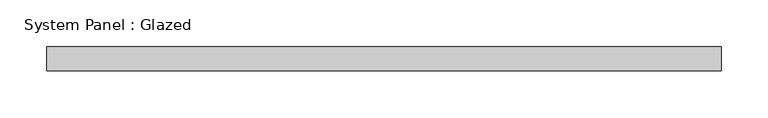
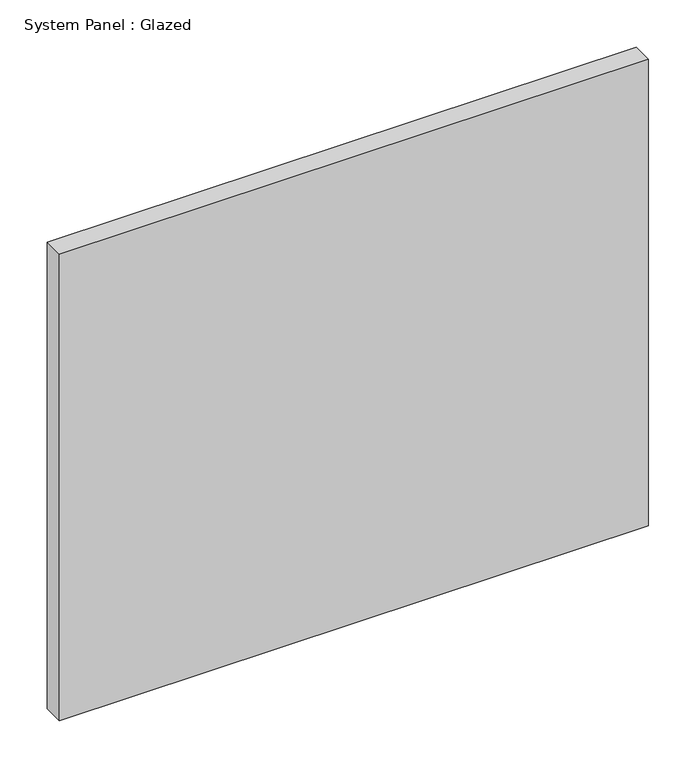
"""IFC4 building model written with IfcOpenShell, lengths in millimetres: plate geometry, System Panel : Glazed."""

from ifc_helpers import new_model, si_unit, origin, origin_with_axes, place, context, project, spatial, polyline, outline, extrude, source, transform, mapped, element, save


def system_panel_glazed_e688d5e8(model_context):
    return source(origin(), model_context, "Body", "SweptSolid", [
        extrude(outline(polyline([(358.775, 19.05), (-358.775, 19.05), (-358.775, 44.45), (358.775, 44.45), (358.775, 19.05)])), origin_with_axes(), (0.0, 0.0, 1.0), 600.9094531),
    ])


if __name__ == "__main__":
    model = new_model("IFC4")
    model_context = context("Model", 3, world=origin())
    ifc_project = project(units=[si_unit("LENGTHUNIT", "METRE", prefix="MILLI")], contexts=[model_context])
    site = spatial("IfcSite", under=ifc_project)
    building = spatial("IfcBuilding", under=site)
    placement = place(None, origin())
    system_panel_glazed_shape = system_panel_glazed_e688d5e8(model_context)
    element("IfcPlate", 1, ObjectType="System Panel : Glazed", at=placement, inside=building, context=model_context, shape_type="MappedRepresentation", body=[
        mapped(system_panel_glazed_shape, transform((0.0, 0.0, 0.0), x_axis=(1.0, 0.0, 0.0), y_axis=(0.0, 1.0, 0.0), z_axis=(0.0, 0.0, 1.0))),
    ])
    save(model, "model.ifc")

# Revit data of these elements
# Type "System Panel : Glazed"
#   Construction Type Id = "GSP4R"
#   Analytic Construction = "1/8 in Pilkington single glazing"
#   Visual Light Transmittance = 0.9
#   Solar Heat Gain Coefficient = 0.86
#   Heat Transfer Coefficient (U) = 1.18115 BTU/(h·ft²·°F)
#   Define Thermal Properties by = 1
# Element 1 (IfcPlate, "System Panel : Glazed")
#   Materials on its faces: "Glass"
# Materials
#   "Glass": class "Glass", colour RGB 0 128 192, transparency 0.75, Description = "Soda Lime Glass", Cost = 0
